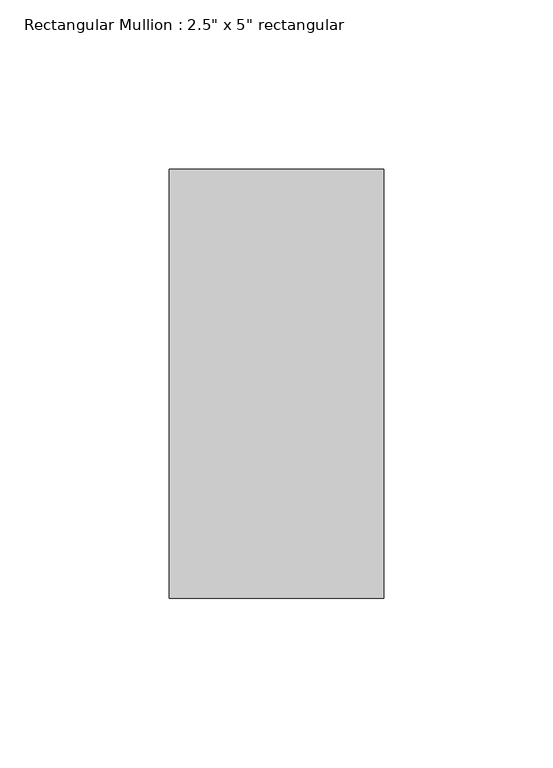
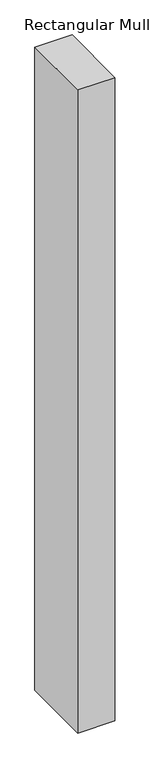
"""IFC4 building model written with IfcOpenShell, lengths in millimetres: member geometry."""

from ifc_helpers import new_model, si_unit, frame, origin, place, context, project, spatial, polyline, outline, extrude, source, transform, mapped, element, save


def member_d74631f0(model_context):
    return source(origin(), model_context, "Body", "SweptSolid", [
        extrude(outline(polyline([(0.0, 63.5), (0.0, -63.5), (-63.5, -63.5), (-63.5, 63.5), (0.0, 63.5)])), frame((0.0, 0.0, -1162.1943025), z_axis=(0.0, 0.0, 1.0), x_axis=(1.0, 0.0, 0.0)), (0.0, 0.0, 1.0), 1162.1943025),
    ])


if __name__ == "__main__":
    model = new_model("IFC4")
    model_context = context("Model", 3, world=origin())
    ifc_project = project(units=[si_unit("LENGTHUNIT", "METRE", prefix="MILLI")], contexts=[model_context])
    site = spatial("IfcSite", under=ifc_project)
    building = spatial("IfcBuilding", under=site)
    placement = place(None, origin())
    member_shape = member_d74631f0(model_context)
    element("IfcMember", 1, ObjectType="Rectangular Mullion : 2.5\" x 5\" rectangular", at=placement, inside=building, context=model_context, shape_type="MappedRepresentation", body=[
        mapped(member_shape, transform((0.0, 0.0, 0.0), x_axis=(1.0, 0.0, 0.0), y_axis=(0.0, 1.0, 0.0), z_axis=(0.0, 0.0, 1.0))),
    ])
    save(model, "model.ifc")

# Revit data of these elements
# Type "Rectangular Mullion : 2.5\" x 5\" rectangular"
#   built-in parameter 1007304 = 0.416667 (stored number, unit not read)
#   built-in parameter 1007301 = 0.104167 (stored number, unit not read)
#   built-in parameter 1007300 = 0.104167 (stored number, unit not read)
# Element 1 (IfcMember, "Rectangular Mullion : 2.5\" x 5\" rectangular")
#   Materials on its faces: "Aluminum"
# Materials
#   "Aluminum": class "Metal", colour RGB 247 247 247, transparency 0, Description = "Aluminum 6061", Cost = 0
